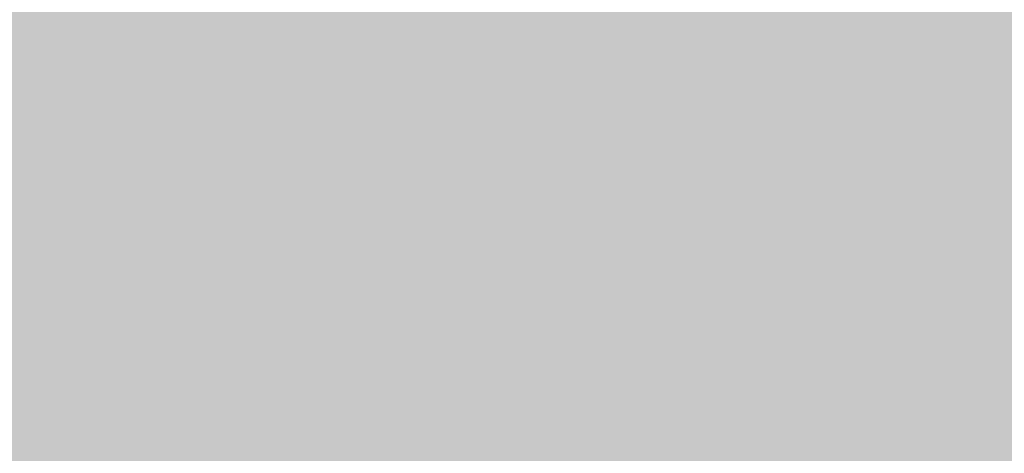
# Model space of a CAD drawing. Units: feet. Extents: x 3168 to 4724, y 827 to 1477.
# Tile 110 of 256: x 3284.48 to 3298.68, y 1087.4 to 1093.65. Entities that reach past the tile are written whole.
import ezdxf

# ---------------------------------------------------------------- set-up
doc = ezdxf.new("R2010")
doc.units = ezdxf.units.FT
doc.layers.add('A-ELEV-PATT', color=8, linetype='Continuous', lineweight=13)

msp = doc.modelspace()

# ---------------------------------------------------------------- hatches: boundary and pattern name
at = {"layer": 'A-ELEV-PATT'}
h = msp.add_hatch(color=256, dxfattribs=at)
h.dxf.hatch_style = 1
edge = h.paths.add_edge_path()
edge.add_ellipse((3552.906, 979.22), major_axis=(36.745, 0), ratio=0.484848, start_angle=0, end_angle=360)
edge = h.paths.add_edge_path()
edge.add_ellipse((3559.892, 929.252), major_axis=(36.745, 0), ratio=0.484848, start_angle=0, end_angle=360)
edge = h.paths.add_edge_path()
edge.add_line((3299.317, 1198.606), (3479.917, 1198.606))
edge.add_line((3479.917, 1198.606), (3479.917, 1209.869))
edge.add_spline(control_points=[(3479.917, 1209.869), (3464.301, 1209.869), (3448.686, 1209.869), (3410.949, 1209.869), (3388.828, 1209.869), (3355.647, 1209.869), (3344.586, 1209.869), (3327.996, 1209.869), (3322.466, 1209.869), (3314.17, 1209.869), (3311.405, 1209.869), (3307.257, 1209.869), (3305.875, 1209.869), (3303.801, 1209.869), (3303.11, 1209.869), (3302.073, 1209.869), (3301.727, 1209.869), (3301.209, 1209.869), (3301.036, 1209.869), (3300.777, 1209.869), (3300.69, 1209.869), (3300.561, 1209.869), (3300.517, 1209.869), (3300.453, 1209.869), (3300.431, 1209.869), (3300.399, 1209.869), (3300.388, 1209.869), (3300.366, 1209.869), (3300.346, 1209.869), (3300.346, 1209.869), (3300.346, 1209.869), (3300.343, 1209.869), (3300.341, 1209.869), (3300.338, 1209.869), (3300.337, 1209.869), (3300.334, 1209.869), (3300.332, 1209.869), (3300.326, 1209.869), (3300.321, 1209.869), (3300.311, 1209.869), (3300.306, 1209.869), (3300.291, 1209.869), (3300.28, 1209.869), (3300.232, 1209.869), (3300.195, 1209.869), (3299.951, 1209.871), (3299.745, 1209.874), (3299.437, 1209.883), (3299.334, 1209.887), (3299.181, 1209.893), (3299.13, 1209.895), (3298.652, 1209.917), (3298.229, 1209.946), (3297.602, 1210.002), (3297.393, 1210.023), (3297.083, 1210.058), (3296.979, 1210.07), (3296.293, 1210.155), (3295.718, 1210.243), (3294.869, 1210.399), (3294.588, 1210.454), (3294.169, 1210.543), (3294.03, 1210.574), (3291.707, 1211.101), (3289.654, 1211.813), (3285.776, 1213.564), (3283.951, 1214.603), (3280.512, 1216.98), (3278.897, 1218.318), (3276.38, 1220.829), (3275.416, 1221.918), (3274.039, 1223.708), (3273.581, 1224.35), (3273.143, 1225.016)], knot_values=[39.119033, 39.119033, 39.119033, 39.119033, 39.286353, 39.286353, 39.523379, 39.523379, 39.641892, 39.641892, 39.701148, 39.701148, 39.730777, 39.730777, 39.745591, 39.745591, 39.752998, 39.752998, 39.756701, 39.756701, 39.758553, 39.758553, 39.759479, 39.759479, 39.759942, 39.759942, 39.760173, 39.760173, 39.760289, 39.760289, 39.760405, 39.760405, 39.760463, 39.760463, 39.763389, 39.763389, 39.764851, 39.764851, 39.767304, 39.767304, 39.773825, 39.773825, 39.78057, 39.78057, 39.79477, 39.79477, 39.845194, 39.845194, 40.126715, 40.126715, 40.267476, 40.267476, 40.337856, 40.337856, 40.927023, 40.927023, 41.221606, 41.221606, 41.368898, 41.368898, 42.202622, 42.202622, 42.619485, 42.619485, 42.827916, 42.827916, 46.118323, 46.118323, 49.408731, 49.408731, 52.699139, 52.699139, 54.927489, 54.927489, 56.104228, 56.104228, 56.104228, 56.104228], weights=[1, 1, 1, 1, 1, 1, 1, 1, 1, 1, 1, 1, 1, 1, 1, 1, 1, 1, 1, 1, 1, 1, 1, 1, 1, 1, 1, 1, 1, 1, 1, 1, 1, 1, 1, 1, 1, 1, 1, 1, 1, 1, 1, 1, 1, 1, 1, 1, 1, 1, 1, 1, 1, 1, 1, 1, 1, 1, 1, 1, 1, 1, 1, 1, 1, 1, 1, 1, 1, 1, 1, 1, 1, 1], degree=3, periodic=0)
edge.add_line((3273.143, 1225.016), (3273.143, 1099.016))
edge.add_line((3273.143, 1099.016), (3299.317, 1099.016))
edge.add_line((3299.317, 1099.016), (3299.317, 1198.606))
edge = h.paths.add_edge_path()
edge.add_line((3304.758, 1324.158), (3479.917, 1324.158))
edge.add_line((3479.917, 1324.158), (3479.917, 1335.715))
edge.add_line((3479.917, 1335.715), (3269.162, 1335.715))
edge.add_spline(control_points=[(3269.162, 1335.715), (3264.024, 1335.715), (3258.364, 1328.958), (3259.264, 1323.9)], knot_values=[0, 0, 0, 0, 15.412191, 15.412191, 15.412191, 15.412191], degree=3, periodic=0)
edge.add_line((3259.264, 1323.9), (3265.517, 1288.769))
edge.add_line((3265.517, 1288.769), (3275.265, 1261.546))
edge.add_line((3275.265, 1261.546), (3304.758, 1261.546))
edge.add_line((3304.758, 1261.546), (3304.758, 1324.158))
h = msp.add_hatch(color=256, dxfattribs=at)
h.dxf.hatch_style = 1
h.paths.add_polyline_path([(3384.525, 1099.016), (3335.029, 1099.016), (3299.317, 1099.016), (3273.143, 1099.016), (3217.565, 1099.016), (3168.069, 827.116), (3335.029, 827.116)])

doc.saveas('drawing.dxf')
